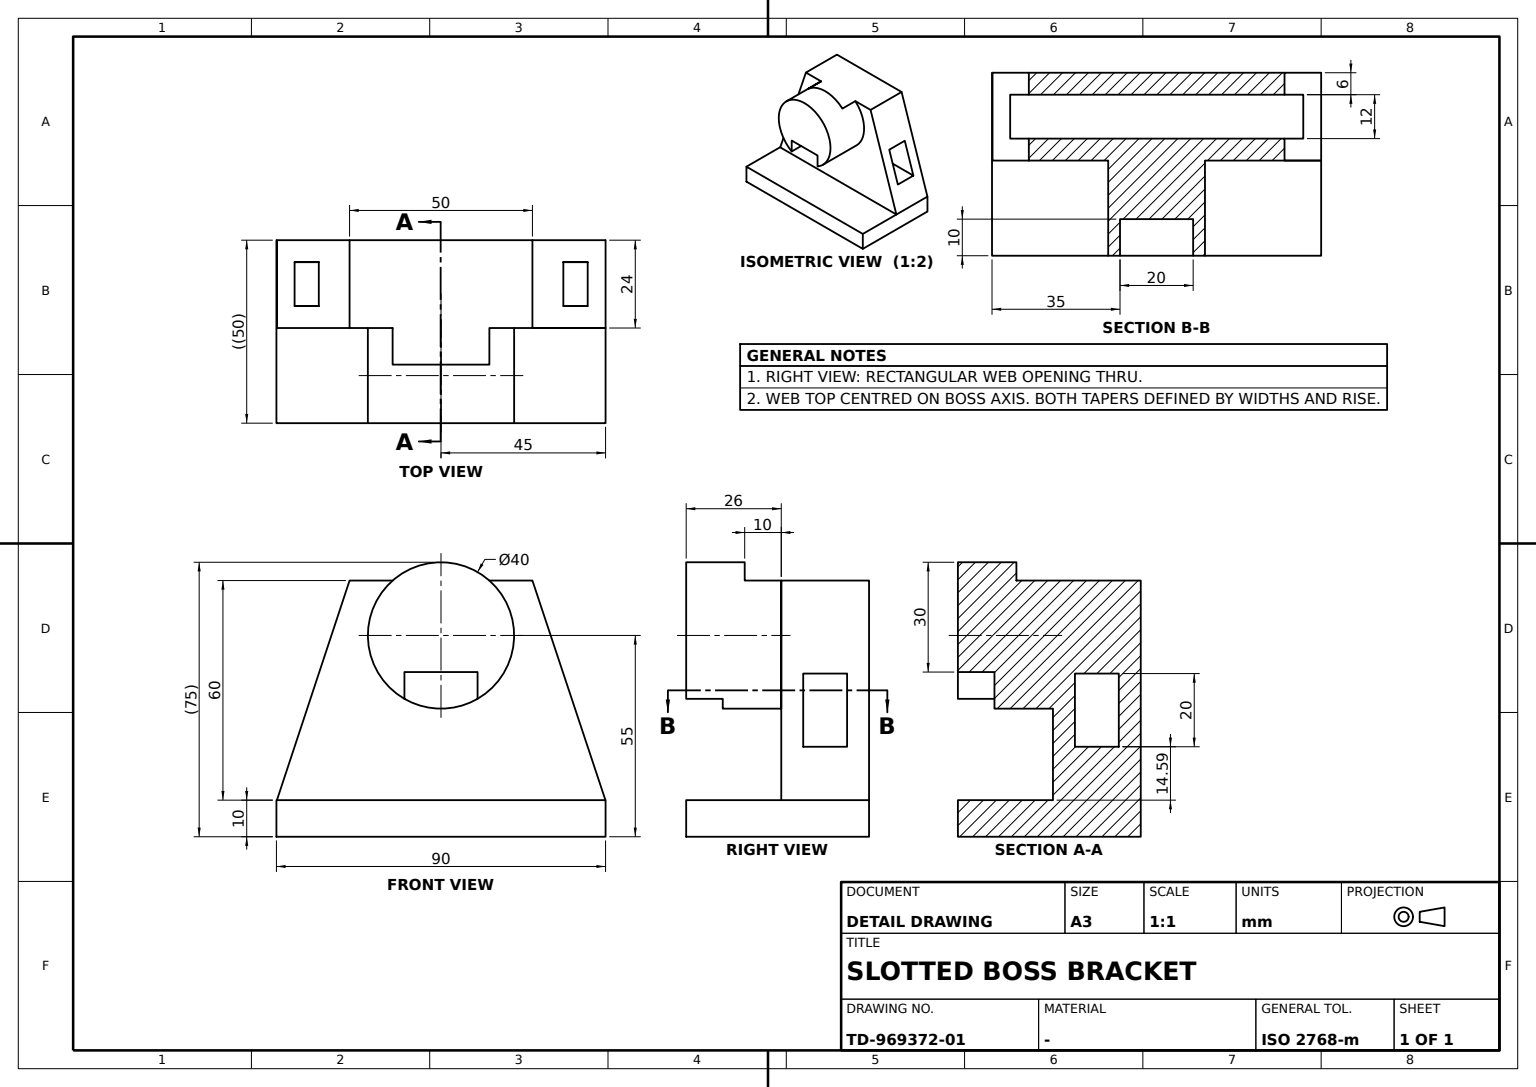
CATIA V5 part; units mm, degrees
sketch "Sketch1" plane through (0, 0, 0) normal (0, 0, 1) x (0, 1, 0)
  line L0 (0, 0) -> (50, 0)
  line L1 (50, 0) -> (50, -90)
  line L2 (50, -90) -> (0, -90)
  line L3 (0, -90) -> (0, 0)
  dimension "length L1" = 90
  dimension "length L0" = 50
  constraint horizontal L0 x-axis
  constraint horizontal L2 x-axis
  constraint vertical L1 y-axis
  constraint vertical L3 y-axis
extrude "Pad1" add sketch "Sketch1" along normal blind 10
sketch "Sketch2" plane through (0, 0, 0) normal (0, -1, 0) x (1, 0, 0)
  line L0 (20, 70) -> (70, 70)
  line L1 (0, 10) -> (90, 10) construction
  line L2 (20, 70) -> (0, 9.8925)
  point P0 (0, 9.8925)
  line L3 (0, 9.8925) -> (89.8989, 9.8925)
  line L4 (89.8989, 9.8925) -> (70, 70)
  dimension "length L0" = 50
  dimension "distance L0 L1" = 60
  constraint horizontal L0 x-axis
  constraint horizontal L3 x-axis
  constraint coincidence P0 y-axis
extrude "Pad2" add sketch "Sketch2" against normal blind 24
sketch "Sketch3" plane through (90, 0, 0) normal (1, 0, 0) x (0, 1, 0)
  line L0 (6, 44.5872) -> (18, 44.5872)
  line L1 (18, 44.5872) -> (18, 24.5872)
  line L2 (18, 24.5872) -> (6, 24.5872)
  line L3 (6, 24.5872) -> (6, 44.5872)
  line L4 (24, 9.8925) -> (24, 70) construction
  dimension "length L1" = 20
  dimension "D2" = 15
  dimension "length L0" = 12
  dimension "distance L1 L4" = 6
  constraint horizontal L0 x-axis
  constraint horizontal L2 x-axis
  constraint vertical L1 y-axis
  constraint vertical L3 y-axis
extrude "Pocket1" cut sketch "Sketch3" against normal up to next
sketch "Sketch4" plane through (0, 24, 0) normal (0, 1, 0) x (-1, 0, 0)
  circle A0 centre (-45, 55) radius 20
  point P0 (-45, 55)
  dimension "radius A0" = 20
  dimension "D2" = 55
  dimension "distance P0 y axis" = 45
extrude "Pad3" add sketch "Sketch4" along normal blind 26
sketch "Sketch5" plane through (0, 50, 0) normal (0, 1, 0) x (-1, 0, 0)
  line L0 (-55, 45) -> (-35, 45)
  line L1 (-35, 45) -> (-35, 32.0977)
  line L2 (-35, 32.0977) -> (-55, 32.0977)
  line L3 (-55, 32.0977) -> (-55, 45)
  line L4 (-90, 0) -> (0, 0) construction
  dimension "length L0" = 20
  dimension "distance L0 L4" = 45
  constraint horizontal L0 x-axis
  constraint horizontal L2 x-axis
  constraint vertical L1 y-axis
  constraint vertical L3 y-axis
extrude "Pocket2" cut sketch "Sketch5" against normal blind 10
sketch "Sketch6" plane through (0, 24, 0) normal (0, -1, 0) x (1, 0, 0)
  line L0 (30, 75.559) -> (60, 75.559)
  line L1 (60, 75.559) -> (60, 70)
  line L2 (60, 70) -> (30, 70)
  line L3 (30, 70) -> (30, 75.559)
  line L4 (70, 70) -> (20, 70) construction
  dimension "length L0" = 30
  constraint horizontal L0 x-axis
  constraint horizontal L2 x-axis
  constraint vertical L1 y-axis
  constraint vertical L3 y-axis
  constraint coincidence L2 L4
extrude "Pocket3" cut sketch "Sketch6" against normal blind 10
properties part number "catia 15"
